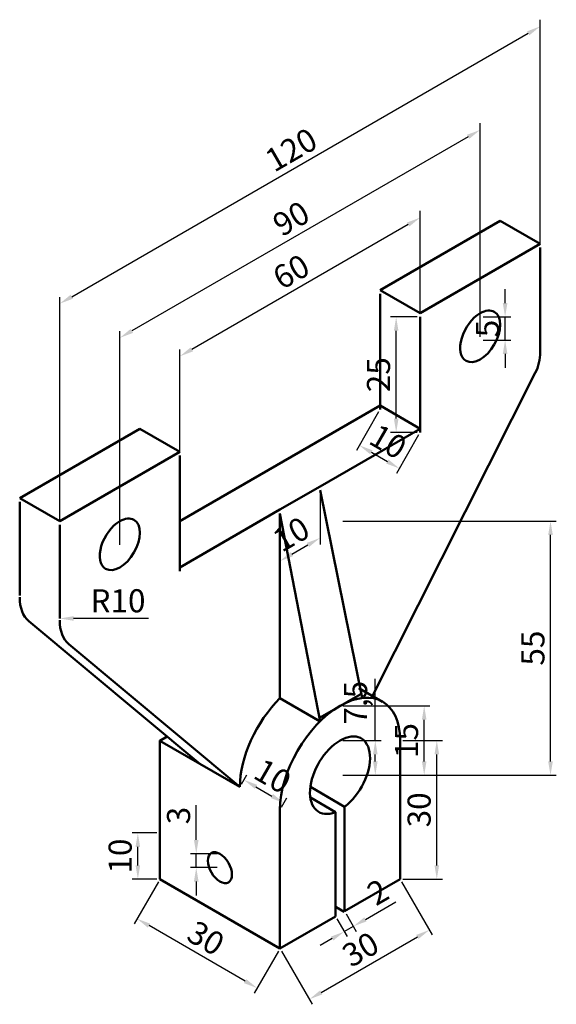
# Model space of a CAD drawing. Units: millimetres. Extents: x -4 to 112, y 13 to 226.
import ezdxf

# ---------------------------------------------------------------- set-up
doc = ezdxf.new("R2010")
doc.units = ezdxf.units.MM
doc.layers.add('M-DIMS', color=2, linetype='Continuous', lineweight=25)
doc.layers.add('M-OUTL', color=7, linetype='Continuous', lineweight=50)
doc.styles.get("Standard").update_dxf_attribs({"font": 'arial.ttf'})
doc.dimstyles.new('ISO-25', dxfattribs={"dimtxt": 5, "dimasz": 3, "dimexe": 1.25, "dimexo": 0.625, "dimtad": 1, "dimtxsty": 'Standard', "dimcen": 2.5, "dimadec": 0, "dimazin": 0, "dimtfac": 1, "dimtmove": 0, "dimatfit": 3, "dimfxl": 1, "dimarcsym": 0})

# ---------------------------------------------------------------- blocks, each defined once
blk = doc.blocks.new('*D1')
at = {"layer": 'Defpoints', "color": 0, "transparency": 16777216}
for p in [(77, 161.76), (82.18, 161.76), (82.18, 136.76)]:
    blk.add_point(p, dxfattribs=at)
at = {"layer": 'M-DIMS', "color": 0, "lineweight": -2, "transparency": 16777216}
for p, q in [((81.55, 161.76), (75.75, 161.76)), ((77, 139.76), (77, 158.76)), ((81.55, 136.76), (75.75, 136.76))]:
    blk.add_line(p, q, dxfattribs=at)
at = {"layer": 'M-DIMS', "color": 0, "transparency": 16777216}
for points in [[(76.5, 158.76), (77.5, 158.76), (77, 161.76)], [(76.5, 139.76), (77.5, 139.76), (77, 136.76)]]:
    blk.add_solid(points, dxfattribs=at)
at = {"layer": 'M-DIMS', "color": 0, "transparency": 16777216, "insert": (73.83, 149.26), "char_height": 5, "attachment_point": 5, "rotation": 90}
blk.add_mtext('25', dxfattribs=at)
blk = doc.blocks.new('*D2')
at = {"layer": 'Defpoints', "color": 0, "transparency": 16777216}
for p in [(95.17, 161.76), (100.56, 161.76), (95.17, 156.76)]:
    blk.add_point(p, dxfattribs=at)
at = {"layer": 'M-DIMS', "color": 0, "lineweight": -2, "transparency": 16777216}
for p, q in [((100.56, 164.76), (100.56, 167.76)), ((95.79, 161.76), (101.81, 161.76)), ((100.56, 156.76), (100.56, 161.76)), ((95.79, 156.76), (101.81, 156.76)), ((100.56, 153.76), (100.56, 150.76))]:
    blk.add_line(p, q, dxfattribs=at)
at = {"layer": 'M-DIMS', "color": 0, "transparency": 16777216}
for points in [[(100.06, 164.76), (101.06, 164.76), (100.56, 161.76)], [(100.06, 153.76), (101.06, 153.76), (100.56, 156.76)]]:
    blk.add_solid(points, dxfattribs=at)
at = {"layer": 'M-DIMS', "color": 0, "transparency": 16777216, "insert": (97.39, 159.26), "char_height": 5, "attachment_point": 5, "rotation": 90}
blk.add_mtext('5', dxfattribs=at)
blk = doc.blocks.new('*D3')
at = {"layer": 'Defpoints', "color": 0, "transparency": 16777216}
for p in [(17.23, 157.23), (95.17, 156.76), (17.23, 111.76)]:
    blk.add_point(p, dxfattribs=at)
at = {"layer": 'M-DIMS', "color": 0, "lineweight": -2, "transparency": 16777216}
for p, q in [((95.17, 157.48), (95.17, 203.68)), ((92.57, 200.73), (19.82, 158.73)), ((17.23, 112.48), (17.23, 158.68))]:
    blk.add_line(p, q, dxfattribs=at)
at = {"layer": 'M-DIMS', "color": 0, "transparency": 16777216}
for points in [[(92.32, 201.17), (92.82, 200.3), (95.17, 202.23)], [(19.57, 159.17), (20.07, 158.3), (17.23, 157.23)]]:
    blk.add_solid(points, dxfattribs=at)
at = {"layer": 'M-DIMS', "color": 0, "transparency": 16777216, "insert": (54.61, 182.49), "char_height": 5, "attachment_point": 5, "rotation": 30}
blk.add_mtext('90', dxfattribs=at)
blk = doc.blocks.new('*D4')
at = {"layer": 'Defpoints', "color": 0, "transparency": 16777216}
for p in [(82.18, 161.76), (30.22, 153.25), (30.22, 131.76)]:
    blk.add_point(p, dxfattribs=at)
at = {"layer": 'M-DIMS', "color": 0, "lineweight": -2, "transparency": 16777216}
for p, q in [((82.18, 162.48), (82.18, 184.69)), ((79.58, 181.75), (32.81, 154.75)), ((30.22, 132.48), (30.22, 154.69))]:
    blk.add_line(p, q, dxfattribs=at)
at = {"layer": 'M-DIMS', "color": 0, "transparency": 16777216}
for points in [[(79.33, 182.18), (79.83, 181.31), (82.18, 183.25)], [(32.56, 155.18), (33.06, 154.31), (30.22, 153.25)]]:
    blk.add_solid(points, dxfattribs=at)
at = {"layer": 'M-DIMS', "color": 0, "transparency": 16777216, "insert": (54.61, 171), "char_height": 5, "attachment_point": 5, "rotation": 30}
blk.add_mtext('60', dxfattribs=at)
blk = doc.blocks.new('*D5')
at = {"layer": 'Defpoints', "color": 0, "transparency": 16777216}
for p in [(108.16, 224.63), (108.16, 176.76), (4.24, 116.76)]:
    blk.add_point(p, dxfattribs=at)
at = {"layer": 'M-DIMS', "color": 0, "lineweight": -2, "transparency": 16777216}
for p, q in [((108.16, 177.48), (108.16, 226.07)), ((6.83, 166.13), (105.56, 223.13)), ((4.24, 117.48), (4.24, 166.07))]:
    blk.add_line(p, q, dxfattribs=at)
at = {"layer": 'M-DIMS', "color": 0, "transparency": 16777216}
for points in [[(105.31, 223.56), (105.81, 222.7), (108.16, 224.63)], [(6.58, 166.56), (7.08, 165.7), (4.24, 164.63)]]:
    blk.add_solid(points, dxfattribs=at)
at = {"layer": 'M-DIMS', "color": 0, "transparency": 16777216, "insert": (54.61, 197.38), "char_height": 5, "attachment_point": 5, "rotation": 30}
blk.add_mtext('120', dxfattribs=at)
blk = doc.blocks.new('*D6')
at = {"layer": 'Defpoints', "color": 0, "transparency": 16777216}
for p in [(64.86, 70.11), (72.49, 70.11), (64.86, 62.61)]:
    blk.add_point(p, dxfattribs=at)
at = {"layer": 'M-DIMS', "color": 0, "lineweight": -2, "transparency": 16777216}
for p, q in [((72.49, 70.11), (72.49, 83.46)), ((65.48, 70.11), (73.74, 70.11)), ((72.49, 65.61), (72.49, 67.11)), ((65.48, 62.61), (73.74, 62.61))]:
    blk.add_line(p, q, dxfattribs=at)
at = {"layer": 'M-DIMS', "color": 0, "transparency": 16777216}
for points in [[(71.99, 67.11), (72.99, 67.11), (72.49, 70.11)], [(71.99, 65.61), (72.99, 65.61), (72.49, 62.61)]]:
    blk.add_solid(points, dxfattribs=at)
at = {"layer": 'M-DIMS', "color": 0, "transparency": 16777216, "insert": (68.87, 78.29), "char_height": 5, "attachment_point": 5, "rotation": 90}
blk.add_mtext('7,5', dxfattribs=at)
blk = doc.blocks.new('*D7')
at = {"layer": 'Defpoints', "color": 0, "transparency": 16777216}
for p in [(64.86, 77.61), (83.06, 77.61), (64.86, 62.61)]:
    blk.add_point(p, dxfattribs=at)
at = {"layer": 'M-DIMS', "color": 0, "lineweight": -2, "transparency": 16777216}
for p, q in [((65.48, 77.61), (84.31, 77.61)), ((83.06, 65.61), (83.06, 74.61)), ((65.48, 62.61), (84.31, 62.61))]:
    blk.add_line(p, q, dxfattribs=at)
at = {"layer": 'M-DIMS', "color": 0, "transparency": 16777216}
for points in [[(82.56, 74.61), (83.56, 74.61), (83.06, 77.61)], [(82.56, 65.61), (83.56, 65.61), (83.06, 62.61)]]:
    blk.add_solid(points, dxfattribs=at)
at = {"layer": 'M-DIMS', "color": 0, "transparency": 16777216, "insert": (79.88, 70.11), "char_height": 5, "attachment_point": 5, "rotation": 90}
blk.add_mtext('15', dxfattribs=at)
blk = doc.blocks.new('*D8')
at = {"layer": 'Defpoints', "color": 0, "transparency": 16777216}
for p in [(77.85, 70.11), (85.79, 70.11), (77.85, 40.11)]:
    blk.add_point(p, dxfattribs=at)
at = {"layer": 'M-DIMS', "color": 0, "lineweight": -2, "transparency": 16777216}
for p, q in [((78.47, 70.11), (87.04, 70.11)), ((85.79, 43.11), (85.79, 67.11)), ((78.47, 40.11), (87.04, 40.11))]:
    blk.add_line(p, q, dxfattribs=at)
at = {"layer": 'M-DIMS', "color": 0, "transparency": 16777216}
for points in [[(85.29, 67.11), (86.29, 67.11), (85.79, 70.11)], [(85.29, 43.11), (86.29, 43.11), (85.79, 40.11)]]:
    blk.add_solid(points, dxfattribs=at)
at = {"layer": 'M-DIMS', "color": 0, "transparency": 16777216, "insert": (82.61, 55.11), "char_height": 5, "attachment_point": 5, "rotation": 90}
blk.add_mtext('30', dxfattribs=at)
blk = doc.blocks.new('*D9')
at = {"layer": 'Defpoints', "color": 0, "transparency": 16777216}
for p in [(77.85, 40.11), (84.19, 29.12), (51.87, 25.11)]:
    blk.add_point(p, dxfattribs=at)
at = {"layer": 'M-DIMS', "color": 0, "lineweight": -2, "transparency": 16777216}
for p, q in [((78.16, 39.57), (84.82, 28.04)), ((60.81, 15.62), (81.59, 27.62)), ((52.18, 24.57), (58.84, 13.04))]:
    blk.add_line(p, q, dxfattribs=at)
at = {"layer": 'M-DIMS', "color": 0, "transparency": 16777216}
for points in [[(81.34, 28.06), (81.84, 27.19), (84.19, 29.12)], [(60.56, 16.06), (61.06, 15.19), (58.21, 14.12)]]:
    blk.add_solid(points, dxfattribs=at)
at = {"layer": 'M-DIMS', "color": 0, "transparency": 16777216, "insert": (69.61, 24.38), "char_height": 5, "attachment_point": 5, "rotation": 30}
blk.add_mtext('30', dxfattribs=at)
blk = doc.blocks.new('*D10')
at = {"layer": 'Defpoints', "color": 0, "transparency": 16777216}
for p in [(63.86, 32.04), (65.86, 33.19), (67.75, 29.92)]:
    blk.add_point(p, dxfattribs=at)
at = {"layer": 'M-DIMS', "color": 0, "lineweight": -2, "transparency": 16777216}
for p, q in [((70.35, 31.42), (76.9, 35.2)), ((66.17, 32.65), (68.37, 28.83)), ((64.17, 31.5), (66.37, 27.68)), ((65.75, 28.76), (67.75, 29.92)), ((63.15, 27.26), (60.55, 25.76))]:
    blk.add_line(p, q, dxfattribs=at)
at = {"layer": 'M-DIMS', "color": 0, "transparency": 16777216}
for points in [[(70.1, 31.85), (70.6, 30.98), (67.75, 29.92)], [(62.9, 27.69), (63.4, 26.83), (65.75, 28.76)]]:
    blk.add_solid(points, dxfattribs=at)
at = {"layer": 'M-DIMS', "color": 0, "transparency": 16777216, "insert": (73.35, 36.77), "char_height": 5, "attachment_point": 5, "rotation": 30}
blk.add_mtext('2', dxfattribs=at)
blk = doc.blocks.new('*D11')
at = {"layer": 'Defpoints', "color": 0, "transparency": 16777216}
for p in [(25.89, 40.11), (20.95, 31.56), (51.87, 25.11)]:
    blk.add_point(p, dxfattribs=at)
at = {"layer": 'M-DIMS', "color": 0, "lineweight": -2, "transparency": 16777216}
for p, q in [((25.57, 39.57), (20.32, 30.48)), ((44.33, 18.06), (23.55, 30.06)), ((51.55, 24.57), (46.3, 15.48))]:
    blk.add_line(p, q, dxfattribs=at)
at = {"layer": 'M-DIMS', "color": 0, "transparency": 16777216}
for points in [[(23.8, 30.49), (23.3, 29.63), (20.95, 31.56)], [(44.58, 18.49), (44.08, 17.63), (46.93, 16.56)]]:
    blk.add_solid(points, dxfattribs=at)
at = {"layer": 'M-DIMS', "color": 0, "transparency": 16777216, "insert": (35.53, 26.81), "char_height": 5, "attachment_point": 5, "rotation": 330}
blk.add_mtext('30', dxfattribs=at)
blk = doc.blocks.new('*D12')
at = {"layer": 'Defpoints', "color": 0, "transparency": 16777216}
for p in [(33.76, 45.61), (38.88, 45.61), (38.88, 42.61)]:
    blk.add_point(p, dxfattribs=at)
at = {"layer": 'M-DIMS', "color": 0, "lineweight": -2, "transparency": 16777216}
for p, q in [((33.76, 48.61), (33.76, 56.14)), ((38.25, 45.61), (32.51, 45.61)), ((33.76, 42.61), (33.76, 45.61)), ((38.25, 42.61), (32.51, 42.61)), ((33.76, 39.61), (33.76, 36.61))]:
    blk.add_line(p, q, dxfattribs=at)
at = {"layer": 'M-DIMS', "color": 0, "transparency": 16777216}
for points in [[(33.26, 48.61), (34.26, 48.61), (33.76, 45.61)], [(33.26, 39.61), (34.26, 39.61), (33.76, 42.61)]]:
    blk.add_solid(points, dxfattribs=at)
at = {"layer": 'M-DIMS', "color": 0, "transparency": 16777216, "insert": (30.58, 53.88), "char_height": 5, "attachment_point": 5, "rotation": 90}
blk.add_mtext('3', dxfattribs=at)
blk = doc.blocks.new('*D13')
at = {"layer": 'Defpoints', "color": 0, "transparency": 16777216}
for p in [(21.13, 50.11), (25.89, 50.11), (25.89, 40.11)]:
    blk.add_point(p, dxfattribs=at)
at = {"layer": 'M-DIMS', "color": 0, "lineweight": -2, "transparency": 16777216}
for p, q in [((25.26, 50.11), (19.88, 50.11)), ((21.13, 43.11), (21.13, 47.11)), ((25.26, 40.11), (19.88, 40.11))]:
    blk.add_line(p, q, dxfattribs=at)
at = {"layer": 'M-DIMS', "color": 0, "transparency": 16777216}
for points in [[(20.63, 47.11), (21.63, 47.11), (21.13, 50.11)], [(20.63, 43.11), (21.63, 43.11), (21.13, 40.11)]]:
    blk.add_solid(points, dxfattribs=at)
at = {"layer": 'M-DIMS', "color": 0, "transparency": 16777216, "insert": (17.95, 45.11), "char_height": 5, "attachment_point": 5, "rotation": 90}
blk.add_mtext('10', dxfattribs=at)
blk = doc.blocks.new('*D14')
at = {"layer": 'Defpoints', "color": 0, "transparency": 16777216}
for p in [(60.53, 124.26), (51.87, 119.26), (60.53, 113.94)]:
    blk.add_point(p, dxfattribs=at)
at = {"layer": 'M-DIMS', "color": 0, "lineweight": -2, "transparency": 16777216}
for p, q in [((60.53, 123.53), (60.53, 112.5)), ((51.87, 118.53), (51.87, 107.5)), ((54.46, 110.44), (57.93, 112.44))]:
    blk.add_line(p, q, dxfattribs=at)
at = {"layer": 'M-DIMS', "color": 0, "transparency": 16777216}
for points in [[(57.68, 112.88), (58.18, 112.01), (60.53, 113.94)], [(54.21, 110.88), (54.71, 110.01), (51.87, 108.94)]]:
    blk.add_solid(points, dxfattribs=at)
at = {"layer": 'M-DIMS', "color": 0, "transparency": 16777216, "insert": (54.61, 114.2), "char_height": 5, "attachment_point": 5, "rotation": 30}
blk.add_mtext('10', dxfattribs=at)
blk = doc.blocks.new('*D15')
at = {"layer": 'Defpoints', "color": 0, "transparency": 16777216}
for p in [(73.52, 141.76), (82.18, 136.76), (77.69, 128.98)]:
    blk.add_point(p, dxfattribs=at)
at = {"layer": 'M-DIMS', "color": 0, "lineweight": -2, "transparency": 16777216}
for p, q in [((73.2, 141.22), (68.4, 132.9)), ((81.86, 136.22), (77.06, 127.9)), ((71.63, 132.48), (75.09, 130.48))]:
    blk.add_line(p, q, dxfattribs=at)
at = {"layer": 'M-DIMS', "color": 0, "transparency": 16777216}
for points in [[(71.88, 132.91), (71.38, 132.05), (69.03, 133.98)], [(75.34, 130.91), (74.84, 130.05), (77.69, 128.98)]]:
    blk.add_solid(points, dxfattribs=at)
at = {"layer": 'M-DIMS', "color": 0, "transparency": 16777216, "insert": (74.95, 134.23), "char_height": 5, "attachment_point": 5, "rotation": 330}
blk.add_mtext('10', dxfattribs=at)
blk = doc.blocks.new('*D16')
at = {"layer": 'Defpoints', "color": 0, "transparency": 16777216}
for p in [(4.24, 96.52), (14.24, 96.52)]:
    blk.add_point(p, dxfattribs=at)
at = {"layer": 'M-DIMS', "color": 0, "lineweight": -2, "transparency": 16777216}
blk.add_line((23.42, 96.52), (7.24, 96.52), dxfattribs=at)
at = {"layer": 'M-DIMS', "color": 0, "transparency": 16777216}
blk.add_solid([(7.24, 97.02), (7.24, 96.02), (4.24, 96.52)], dxfattribs=at)
at = {"layer": 'M-DIMS', "color": 0, "transparency": 16777216, "insert": (16.83, 99.7), "char_height": 5, "attachment_point": 5}
blk.add_mtext('R10', dxfattribs=at)
blk = doc.blocks.new('*D17')
at = {"layer": 'Defpoints', "color": 0, "transparency": 16777216}
for p in [(64.86, 117.61), (110.38, 117.61), (64.86, 62.61)]:
    blk.add_point(p, dxfattribs=at)
at = {"layer": 'M-DIMS', "color": 0, "lineweight": -2, "transparency": 16777216}
for p, q in [((65.48, 117.61), (111.63, 117.61)), ((110.38, 65.61), (110.38, 114.61)), ((65.48, 62.61), (111.63, 62.61))]:
    blk.add_line(p, q, dxfattribs=at)
at = {"layer": 'M-DIMS', "color": 0, "transparency": 16777216}
for points in [[(109.88, 114.61), (110.88, 114.61), (110.38, 117.61)], [(109.88, 65.61), (110.88, 65.61), (110.38, 62.61)]]:
    blk.add_solid(points, dxfattribs=at)
at = {"layer": 'M-DIMS', "color": 0, "transparency": 16777216, "insert": (107.22, 90.11), "char_height": 5, "attachment_point": 5, "rotation": 90}
blk.add_mtext('55', dxfattribs=at)
blk = doc.blocks.new('*D18')
at = {"layer": 'Defpoints', "color": 0, "transparency": 16777216}
for p in [(43.21, 60.11), (52.73, 56.6), (51.87, 55.11)]:
    blk.add_point(p, dxfattribs=at)
at = {"layer": 'M-DIMS', "color": 0, "lineweight": -2, "transparency": 16777216}
for p, q in [((43.52, 60.66), (44.69, 62.69)), ((46.67, 60.1), (50.13, 58.1)), ((52.18, 55.66), (53.35, 57.69))]:
    blk.add_line(p, q, dxfattribs=at)
at = {"layer": 'M-DIMS', "color": 0, "transparency": 16777216}
for points in [[(46.92, 60.54), (46.42, 59.67), (44.07, 61.6)], [(50.38, 58.54), (49.88, 57.67), (52.73, 56.6)]]:
    blk.add_solid(points, dxfattribs=at)
at = {"layer": 'M-DIMS', "color": 0, "transparency": 16777216, "insert": (49.99, 61.86), "char_height": 5, "attachment_point": 5, "rotation": 330}
blk.add_mtext('10', dxfattribs=at)

msp = doc.modelspace()

# ---------------------------------------------------------------- linework, layer by layer
at = {"layer": 'M-OUTL'}
for p, q in [((73.517, 167.565), (99.498, 182.565)), ((108.158, 177.565), (99.498, 182.565)), ((82.177, 162.565), (108.158, 177.565)), ((108.158, 154.134), (108.158, 176.756)), ((82.177, 162.565), (73.517, 167.565)), ((73.517, 166.756), (73.517, 141.756)), ((82.177, 136.756), (82.177, 161.756)), ((71.645, 79.322), (107.088, 149.633)), ((30.216, 117.565), (73.517, 142.565)), ((82.177, 137.565), (73.517, 142.565)), ((-4.425, 122.565), (21.556, 137.565)), ((30.216, 132.565), (21.556, 137.565)), ((60.527, 125.065), (82.177, 137.565)), ((4.235, 117.565), (30.216, 132.565)), ((30.216, 106.756), (30.216, 131.756)), ((51.867, 120.065), (60.527, 125.065)), ((60.527, 124.256), (69.644, 79.322)), ((4.235, 117.565), (-4.425, 122.565)), ((-4.425, 121.756), (-4.425, 101.518)), ((30.216, 107.565), (51.867, 120.065)), ((51.867, 79.256), (51.867, 119.256)), ((51.867, 119.256), (60.527, 74.256)), ((4.235, 96.518), (4.235, 116.756)), ((34.546, 65.065), (-2.467, 95.932)), ((43.206, 60.065), (6.193, 90.932)), ((74.043, 78.475), (68.924, 81.43)), ((60.527, 74.256), (51.867, 79.256)), ((69.187, 80.065), (60.527, 75.065)), ((25.886, 70.065), (27.46, 70.974)), ((25.886, 40.114), (25.886, 70.114)), ((34.546, 65.065), (25.886, 70.065)), ((77.847, 40.114), (77.847, 70.114)), ((43.206, 60.065), (34.546, 65.065)), ((65.857, 55.781), (58.439, 60.064)), ((63.857, 54.626), (58.439, 57.754)), ((65.857, 55.781), (65.857, 33.192)), ((51.867, 55.114), (51.867, 25.114)), ((63.857, 54.626), (63.857, 32.037)), ((51.867, 25.114), (25.886, 40.114)), ((65.857, 33.192), (77.847, 40.114)), ((51.867, 25.114), (63.857, 32.037)), ((65.723, 33.065), (63.991, 34.065))]:
    msp.add_line(p, q, dxfattribs=at)
msp.add_arc((98.158, 154.134), 10, 333.24808, 0, dxfattribs=at)
for centre, major_axis, start_param, end_param in [((95.168, 157.565), (3.062, 5.303), 0.7853982, 3.1415927), ((95.168, 157.565), (3.062, 5.303), 3.1415927, 6.2831853), ((95.168, 157.565), (3.062, 5.303), 0, 0.7853982), ((17.226, 112.565), (3.062, 5.303), 0.7853982, 3.1415927), ((17.226, 112.565), (3.062, 5.303), 3.1415927, 6.2831853), ((17.226, 112.565), (3.062, 5.303), 0, 0.7853982), ((4.235, 106.134), (-6.124, -10.607), 5.4977871, 6.1835167), ((12.895, 101.134), (-6.124, -10.607), 5.4977871, 6.1835167), ((64.857, 62.614), (-9.186, -15.91), 2.3561945, 5.4977871), ((56.197, 67.614), (-9.186, -15.91), 4.2668277, 5.4977871), ((64.857, 62.614), (-4.593, -7.955), 0.9399731, 6.9140086)]:
    msp.add_ellipse(centre, major_axis=major_axis, ratio=0.5773503, start_param=start_param, end_param=end_param, dxfattribs=at)
msp.add_ellipse((38.876, 42.614), major_axis=(1.837, -3.182), ratio=0.5773503, dxfattribs=at)

# ---------------------------------------------------------------- dimensions: what is measured, and where the dimension line sits
at = {"layer": 'M-DIMS'}
for p1, p2, distance, picture, middle in [((4.235, 116.756), (108.158, 176.756), 41.46, '*D5', (54.608, 197.382)), ((95.168, 156.756), (17.226, 111.756), -39.385, '*D3', (54.608, 182.487)), ((82.177, 161.756), (30.216, 131.756), -18.612, '*D4', (54.608, 171)), ((73.517, 141.756), (82.177, 136.756), -8.978, '*D15', (74.947, 134.233)), ((51.867, 119.256), (60.527, 124.256), -8.931, '*D14', (54.608, 114.195)), ((43.206, 60.114), (51.867, 55.114), 1.721, '*D18', (49.986, 61.857)), ((51.867, 25.114), (25.886, 40.114), 9.877, '*D11', (35.528, 26.814)), ((51.867, 25.114), (77.847, 40.114), -12.689, '*D9', (69.612, 24.378))]:
    dim = msp.add_aligned_dim(p1=p1, p2=p2, distance=distance, dimstyle='ISO-25', override={"dimclrd": 0, "dimclre": 0, "dimclrt": 0}, dxfattribs=at)
    dim.commit()
    dim.dimension.update_dxf_attribs({"geometry": picture, "text_midpoint": middle})
for base, p1, p2, picture, middle in [((100.562, 161.756), (95.168, 156.756), (95.168, 161.756), '*D2', (97.395, 159.256)), ((77.004, 161.756), (82.177, 136.756), (82.177, 161.756), '*D1', (73.826, 149.256)), ((110.385, 117.614), (64.857, 62.614), (64.857, 117.614), '*D17', (107.217, 90.114)), ((72.492, 70.114), (64.857, 62.614), (64.857, 70.114), '*D6', (68.872, 78.289)), ((83.058, 77.614), (64.857, 62.614), (64.857, 77.614), '*D7', (79.88, 70.114)), ((85.786, 70.114), (77.847, 40.114), (77.847, 70.114), '*D8', (82.607, 55.114)), ((33.763, 45.614), (38.876, 42.614), (38.876, 45.614), '*D12', (30.584, 53.876)), ((21.127, 50.114), (25.886, 40.114), (25.886, 50.114), '*D13', (17.949, 45.114))]:
    dim = msp.add_linear_dim(base=base, p1=p1, p2=p2, angle=90, dimstyle='ISO-25', override={"dimclrd": 0, "dimclre": 0, "dimclrt": 0}, dxfattribs=at)
    dim.commit()
    dim.dimension.update_dxf_attribs({"geometry": picture, "text_midpoint": middle})
dim = msp.add_radius_dim(center=(14.235, 96.518), mpoint=(4.235, 96.518), dimstyle='ISO-25', override={"dimclrd": 0, "dimclre": 0, "dimclrt": 0}, dxfattribs=at)
dim.commit()
dim.dimension.update_dxf_attribs({"geometry": '*D16', "text_midpoint": (16.825, 96.518), "dimtype": 164})
dim = msp.add_aligned_dim(p1=(63.857, 32.037), p2=(65.857, 33.192), distance=-3.783, text='2', dimstyle='ISO-25', override={"dimclrd": 0, "dimclre": 0, "dimclrt": 0}, dxfattribs=at)
dim.commit()
dim.dimension.update_dxf_attribs({"geometry": '*D10', "text_midpoint": (73.352, 36.771)})

doc.saveas('drawing.dxf')
